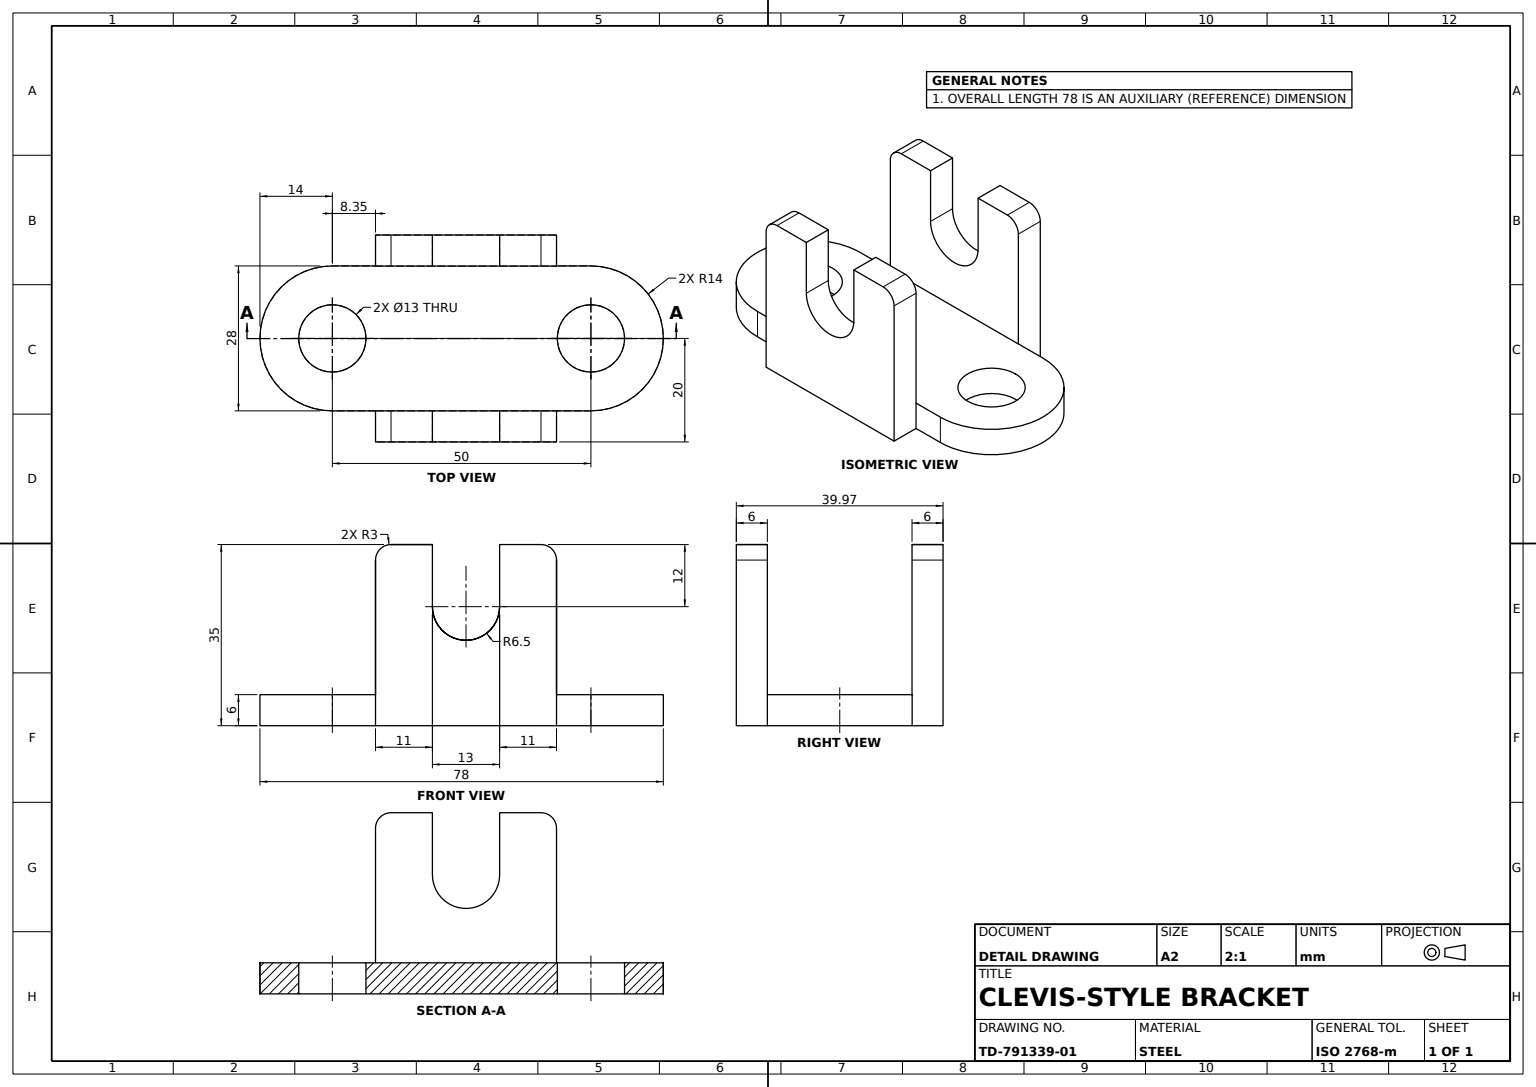
from build123d import *

# Parameters (mm, degrees)
CLEVIS_EAR_1_DEPTH         = 6
BASE_PLATE_DEPTH           = 6
MOUNTING_HOLES_SKETCH_R    = 6.5
MOUNTING_HOLES_2X_13_DEPTH = 67.717997207
CLEVIS_EAR_2_DEPTH         = 6


with BuildPart() as part:
    # Clevis Ear 1 Sketch → Clevis Ear 1 (new body)
    with BuildSketch(Plane.XY):
        with BuildLine():
            Line((-27.211796247, 0), (7.788203753, 0))
            Line((7.788203753, 0), (7.788203753, 32))
            ThreePointArc((7.788203753, 32), (6.909524097, 34.121320344), (4.788203753, 35))
            Line((4.788203753, 35), (-3.211796247, 35))
            Line((-3.211796247, 35), (-3.211796247, 23))
            ThreePointArc((-3.211796247, 23), (-9.711796247, 16.5), (-16.211796247, 23))
            Line((-16.211796247, 23), (-16.211796247, 35))
            Line((-16.211796247, 35), (-24.211796247, 35))
            ThreePointArc((-24.211796247, 35), (-26.33311659, 34.121320344), (-27.211796247, 32))
            Line((-27.211796247, 32), (-27.211796247, 0))
        make_face()
    extrude(amount=CLEVIS_EAR_1_DEPTH)

    # Base Plate Sketch → Base Plate (add)
    with BuildSketch(Plane.XZ):
        with BuildLine():
            Line((-35.558376082, 5.974380222), (14.441623918, 5.974380222))
            ThreePointArc((14.441623918, 5.974380222), (28.441623918, 19.974380222), (14.441623918, 33.974380222))
            Line((14.441623918, 33.974380222), (-35.558376082, 33.974380222))
            ThreePointArc((-35.558376082, 33.974380222), (-49.558376082, 19.974380222), (-35.558376082, 5.974380222))
        make_face()
    extrude(amount=-BASE_PLATE_DEPTH)

    # Mounting Holes Sketch → Mounting Holes 2xØ13 (cut, through all)
    with BuildSketch(Plane(origin=(0, 6, 0), x_dir=(1, 0, 0), z_dir=(0, 1, 0))):
        with Locations(Location((-35.558376082, -19.974380222, 0), (0, 0, 270))):
            Circle(MOUNTING_HOLES_SKETCH_R)
        with Locations(Location((14.441623918, -19.974380222, 0), (0, 0, 270))):
            Circle(MOUNTING_HOLES_SKETCH_R)
    extrude(amount=-MOUNTING_HOLES_2X_13_DEPTH, mode=Mode.SUBTRACT)

    # Clevis Ear 2 Sketch → Clevis Ear 2 (add)
    with BuildSketch(Plane.XY.offset(33.974380222)):
        with BuildLine():
            Line((-27.211796247, 0), (7.788203753, 0))
            Line((7.788203753, 0), (7.788203753, 32))
            ThreePointArc((7.788203753, 32), (6.909524097, 34.121320344), (4.788203753, 35))
            Line((4.788203753, 35), (-3.211796247, 35))
            Line((-3.211796247, 35), (-3.211796247, 23))
            ThreePointArc((-3.211796247, 23), (-9.711796247, 16.5), (-16.211796247, 23))
            Line((-16.211796247, 23), (-16.211796247, 35))
            Line((-16.211796247, 35), (-24.211796247, 35))
            ThreePointArc((-24.211796247, 35), (-26.33311659, 34.121320344), (-27.211796247, 32))
            Line((-27.211796247, 32), (-27.211796247, 0))
        make_face()
    extrude(amount=CLEVIS_EAR_2_DEPTH)


solid = part.part
